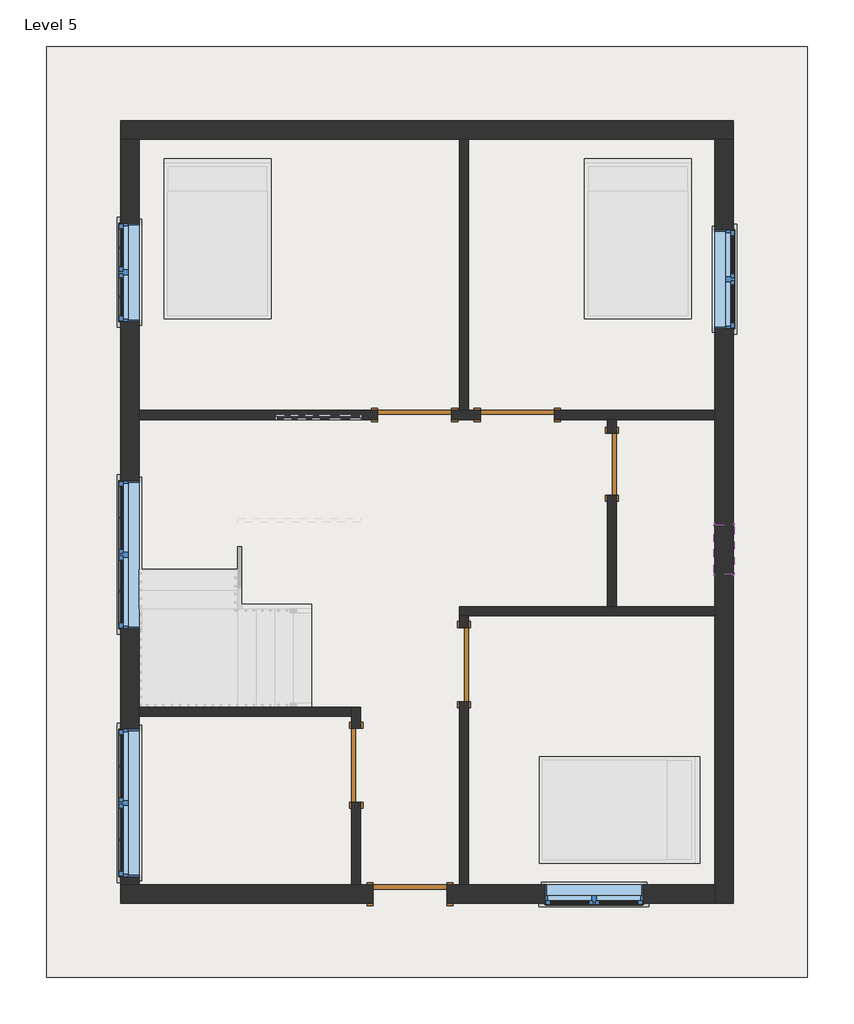
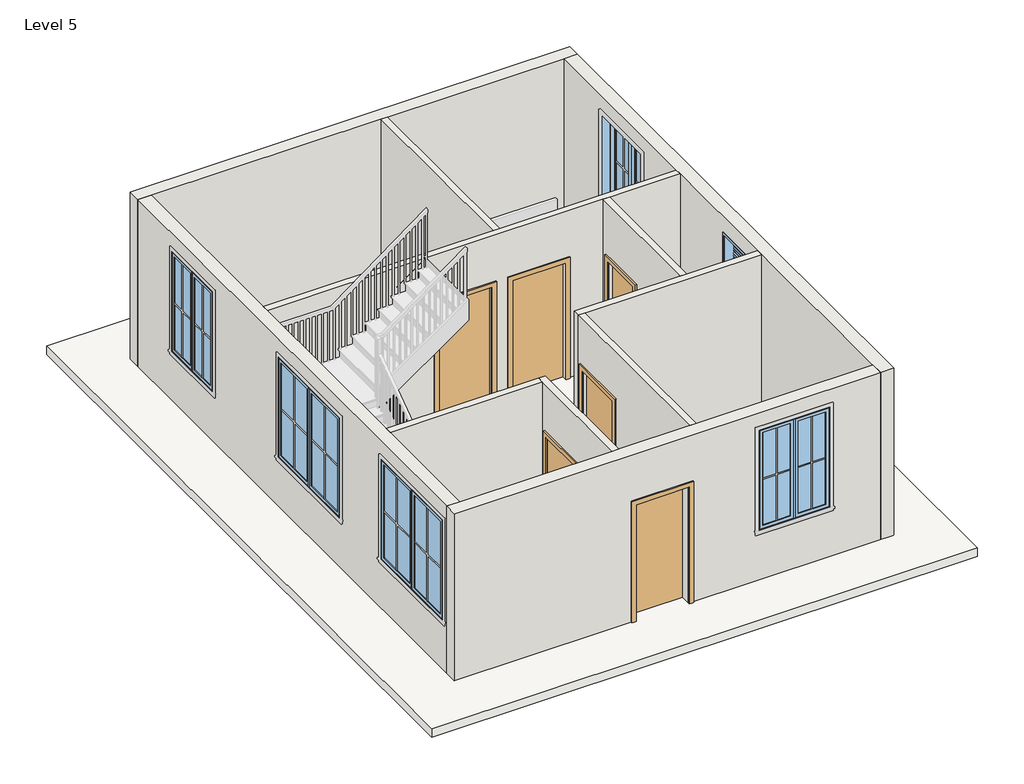
# One storey, part 1 of 3: 11 walls, 6 doors, 6 windows, 1 roof.
"""IFC4 building model written with IfcOpenShell, lengths in millimetres."""

from ifc_helpers import new_model, si_unit, frame, origin, place, context, project, spatial, polyline, outline, extrude, faceted_brep, transform, mapped, element, save
from components import door_f2b275c1, single_flush_door_3_e5f9f3c4, single_flush_door_3_305aa2a5, single_flush_door_3_a90ba1ad, window_casement_double_win_4_6ca1769e, window_casement_double_win_6_ce442eab, window_f2d8fef0

model = new_model("IFC4")

# Units and contexts
model_context = context("Model", 3, world=origin())
ifc_project = project(units=[si_unit("LENGTHUNIT", "METRE", prefix="MILLI")], contexts=[model_context])

# Site, building, storey
site = spatial("IfcSite", under=ifc_project)
building = spatial("IfcBuilding", under=site)
storey = spatial("IfcBuildingStorey", under=building, Name="Level 5", Elevation=12649.2)

# Doors
placement = place(None, origin())
door_shape = door_f2b275c1(model_context)
element("IfcDoor", 1, ObjectType="Single-Flush : 2'6\"", at=placement, inside=storey, context=model_context, shape_type="MappedRepresentation", body=[
    mapped(door_shape, transform((1031.6394609, 262.5126239, 12649.2), x_axis=(0.0, 1.0, 0.0), y_axis=(-1.0, 0.0, 0.0), z_axis=(0.0, 0.0, 1.0))),
])
single_flush_door_3_shape = single_flush_door_3_e5f9f3c4(model_context)
element("IfcDoor", 2, ObjectType="Single-Flush : door 3'", at=placement, inside=storey, context=model_context, shape_type="MappedRepresentation", body=[
    mapped(single_flush_door_3_shape, transform((-1406.7605391, 872.1126239, 12649.2), x_axis=(1.0, 0.0, 0.0), y_axis=(0.0, 1.0, 0.0), z_axis=(0.0, 0.0, 1.0))),
])
element("IfcDoor", 3, ObjectType="Single-Flush : door 3'", at=placement, inside=storey, context=model_context, shape_type="MappedRepresentation", body=[
    mapped(single_flush_door_3_shape, transform((-2130.6605391, -3458.5873761, 12649.2), x_axis=(0.0, 1.0, 0.0), y_axis=(-1.0, 0.0, 0.0), z_axis=(0.0, 0.0, 1.0))),
])
single_flush_door_3_2_shape = single_flush_door_3_305aa2a5(model_context)
element("IfcDoor", 4, ObjectType="Single-Flush : door 3'", at=placement, inside=storey, context=model_context, shape_type="MappedRepresentation", body=[
    mapped(single_flush_door_3_2_shape, transform((-136.7605391, 872.1126239, 12649.2), x_axis=(-1.0, 0.0, 0.0), y_axis=(0.0, -1.0, 0.0), z_axis=(0.0, 0.0, 1.0))),
])
element("IfcDoor", 5, ObjectType="Single-Flush : door 3'", at=placement, inside=storey, context=model_context, shape_type="MappedRepresentation", body=[
    mapped(single_flush_door_3_2_shape, transform((-797.1605391, -2213.9873761, 12649.2), x_axis=(0.0, 1.0, 0.0), y_axis=(-1.0, 0.0, 0.0), z_axis=(0.0, 0.0, 1.0))),
])
single_flush_door_3_3_shape = single_flush_door_3_a90ba1ad(model_context)
element("IfcDoor", 6, ObjectType="Single-Flush : door 3'", at=placement, inside=storey, context=model_context, shape_type="MappedRepresentation", body=[
    mapped(single_flush_door_3_3_shape, transform((-1463.9105391, -5052.4373761, 12649.2), x_axis=(-1.0, 0.0, 0.0), y_axis=(0.0, -1.0, 0.0), z_axis=(0.0, 0.0, 1.0))),
])

# Roof
element("IfcRoof", 7, ObjectType="Generic - 12\"", at=placement, inside=storey, context=model_context, shape_type="SweptSolid", body=[
    extrude(outline(polyline([(-5959.7105391, 5425.0626239), (3450.9894609, 5425.0626239), (3450.9894609, -6081.1373761), (-5959.7105391, -6081.1373761), (-5959.7105391, 5425.0626239)])), frame((0.0, 0.0, 12496.8), z_axis=(0.0, 0.0, 1.0), x_axis=(1.0, 0.0, 0.0)), (0.0, 0.0, 1.0), 152.4),
])

# Walls
element("IfcWall", 8, ObjectType="WALL 4.5\"", at=placement, inside=storey, context=model_context, shape_type="SweptSolid", body=[
    extrude(outline(polyline([(-854.3105391, 929.2626239), (-854.3105391, 4282.0626239), (-740.0105391, 4282.0626239), (-740.0105391, 929.2626239), (-854.3105391, 929.2626239)])), frame((0.0, 0.0, 12649.2), z_axis=(0.0, 0.0, 1.0), x_axis=(1.0, 0.0, 0.0)), (0.0, 0.0, 1.0), 3048.0),
])
element("IfcWall", 9, ObjectType="WALL 4.5\"", at=placement, inside=storey, context=model_context, shape_type="Brep", body=[
    faceted_brep([(-949.5605391, 814.9626239, 12649.2), (-593.9605391, 814.9626239, 12649.2), (-593.9605391, 814.9626239, 14782.8), (320.4394609, 814.9626239, 14782.8), (320.4394609, 814.9626239, 12649.2), (974.4894609, 814.9626239, 12649.2), (1088.7894609, 814.9626239, 12649.2), (2307.9894609, 814.9626239, 12649.2), (2307.9894609, 814.9626239, 15697.2), (1088.7894609, 814.9626239, 15697.2), (974.4894609, 814.9626239, 15697.2), (-4816.7105391, 814.9626239, 15697.2), (-4816.7105391, 814.9626239, 12649.2), (-1863.9605391, 814.9626239, 12649.2), (-1863.9605391, 814.9626239, 14782.8), (-949.5605391, 814.9626239, 14782.8), (-593.9605391, 929.2626239, 14782.8), (-593.9605391, 929.2626239, 12649.2), (-740.0105391, 929.2626239, 12649.2), (-854.3105391, 929.2626239, 12649.2), (-949.5605391, 929.2626239, 12649.2), (-949.5605391, 929.2626239, 14782.8), (-1863.9605391, 929.2626239, 14782.8), (-1863.9605391, 929.2626239, 12649.2), (-4816.7105391, 929.2626239, 12649.2), (-4816.7105391, 929.2626239, 15697.2), (-854.3105391, 929.2626239, 15697.2), (-740.0105391, 929.2626239, 15697.2), (2307.9894609, 929.2626239, 15697.2), (2307.9894609, 929.2626239, 12649.2), (320.4394609, 929.2626239, 12649.2), (320.4394609, 929.2626239, 14782.8)], [[[0, 1, 2, 3, 4, 5, 6, 7, 8, 9, 10, 11, 12, 13, 14, 15]], [[16, 17, 18, 19, 20, 21, 22, 23, 24, 25, 26, 27, 28, 29, 30, 31]], [[13, 12, 24, 23]], [[30, 29, 7, 6, 5, 4]], [[20, 19, 18, 17, 1, 0]], [[8, 7, 29, 28]], [[12, 11, 25, 24]], [[21, 20, 0, 15]], [[22, 21, 15, 14]], [[23, 22, 14, 13]], [[2, 1, 17, 16]], [[3, 2, 16, 31]], [[4, 3, 31, 30]], [[11, 10, 9, 8, 28, 27, 26, 25]]]),
])
element("IfcWall", 10, ObjectType="WALL 4.5\"", at=placement, inside=storey, context=model_context, shape_type="SweptSolid", body=[
    extrude(outline(polyline([(814.9626239, 12649.2), (643.5126239, 12649.2), (643.5126239, 14681.2), (-118.4873761, 14681.2), (-118.4873761, 12649.2), (-1496.4373761, 12649.2), (-1496.4373761, 15697.2), (814.9626239, 15697.2), (814.9626239, 12649.2)])), frame((974.4894609, 0.0, 0.0), z_axis=(1.0, 0.0, 0.0), x_axis=(0.0, 1.0, 0.0)), (0.0, 0.0, 1.0), 114.3),
])
element("IfcWall", 11, ObjectType="WALL 4.5\"", at=placement, inside=storey, context=model_context, shape_type="Brep", body=[
    faceted_brep([(2307.9894609, -1496.4373761, 12649.2), (1088.7894609, -1496.4373761, 12649.2), (974.4894609, -1496.4373761, 12649.2), (-854.3105391, -1496.4373761, 12649.2), (-854.3105391, -1496.4373761, 15697.2), (974.4894609, -1496.4373761, 15697.2), (1088.7894609, -1496.4373761, 15697.2), (2307.9894609, -1496.4373761, 15697.2), (2307.9894609, -1610.7373761, 12649.2), (2307.9894609, -1610.7373761, 15697.2), (-740.0105391, -1610.7373761, 15697.2), (-854.3105391, -1610.7373761, 15697.2), (-854.3105391, -1610.7373761, 12649.2), (-740.0105391, -1610.7373761, 12649.2)], [[[0, 1, 2, 3, 4, 5, 6, 7]], [[8, 9, 10, 11, 12, 13]], [[3, 2, 1, 0, 8, 13, 12]], [[0, 7, 9, 8]], [[4, 3, 12, 11]], [[7, 6, 5, 4, 11, 10, 9]]]),
])
element("IfcWall", 12, ObjectType="WALL 4.5\"", at=placement, inside=storey, context=model_context, shape_type="SweptSolid", body=[
    extrude(outline(polyline([(-1610.7373761, 12649.2), (-1756.7873761, 12649.2), (-1756.7873761, 14782.8), (-2671.1873761, 14782.8), (-2671.1873761, 12649.2), (-4938.1373761, 12649.2), (-4938.1373761, 15697.2), (-1610.7373761, 15697.2), (-1610.7373761, 12649.2)])), frame((-854.3105391, 0.0, 0.0), z_axis=(1.0, 0.0, 0.0), x_axis=(0.0, 1.0, 0.0)), (0.0, 0.0, 1.0), 114.3),
])
element("IfcWall", 13, ObjectType="WALL 4.5\"", at=placement, inside=storey, context=model_context, shape_type="Brep", body=[
    faceted_brep([(-2073.5105391, -3001.3873761, 14782.8), (-2073.5105391, -3001.3873761, 12649.2), (-2073.5105391, -2741.0373761, 12649.2), (-2073.5105391, -2741.0373761, 15697.2), (-2073.5105391, -4938.1373761, 15697.2), (-2073.5105391, -4938.1373761, 12649.2), (-2073.5105391, -3915.7873761, 12649.2), (-2073.5105391, -3915.7873761, 14782.8), (-2187.8105391, -2741.0373761, 12649.2), (-2187.8105391, -2855.3373761, 12649.2), (-2187.8105391, -3001.3873761, 12649.2), (-2187.8105391, -3001.3873761, 14782.8), (-2187.8105391, -3915.7873761, 14782.8), (-2187.8105391, -3915.7873761, 12649.2), (-2187.8105391, -4938.1373761, 12649.2), (-2187.8105391, -4938.1373761, 15697.2), (-2187.8105391, -2855.3373761, 15697.2), (-2187.8105391, -2741.0373761, 15697.2)], [[[0, 1, 2, 3, 4, 5, 6, 7]], [[8, 9, 10, 11, 12, 13, 14, 15, 16, 17]], [[6, 5, 14, 13]], [[2, 1, 10, 9, 8]], [[5, 4, 15, 14]], [[3, 2, 8, 17]], [[11, 10, 1, 0]], [[12, 11, 0, 7]], [[13, 12, 7, 6]], [[4, 3, 17, 16, 15]]]),
])
element("IfcWall", 14, ObjectType="WALL 4.5\"", at=placement, inside=storey, context=model_context, shape_type="SweptSolid", body=[
    extrude(outline(polyline([(-4816.7105391, -2741.0373761), (-2187.8105391, -2741.0373761), (-2187.8105391, -2855.3373761), (-4816.7105391, -2855.3373761), (-4816.7105391, -2741.0373761)])), frame((0.0, 0.0, 12649.2), z_axis=(0.0, 0.0, 1.0), x_axis=(1.0, 0.0, 0.0)), (0.0, 0.0, 1.0), 3048.0),
])
element("IfcWall", 15, ObjectType="WALL 9\"", at=placement, inside=storey, context=model_context, shape_type="Brep", body=[
    faceted_brep([(-5045.3105391, 4282.0626239, 12649.2), (-4816.7105391, 4282.0626239, 12649.2), (-854.3105391, 4282.0626239, 12649.2), (-740.0105391, 4282.0626239, 12649.2), (2307.9894609, 4282.0626239, 12649.2), (2536.5894609, 4282.0626239, 12649.2), (2536.5894609, 4282.0626239, 15697.2), (2307.9894609, 4282.0626239, 15697.2), (-740.0105391, 4282.0626239, 15697.2), (-854.3105391, 4282.0626239, 15697.2), (-4816.7105391, 4282.0626239, 15697.2), (-5045.3105391, 4282.0626239, 15697.2), (-5045.3105391, 4510.6626239, 12649.2), (-5045.3105391, 4510.6626239, 15697.2), (2536.5894609, 4510.6626239, 15697.2), (2536.5894609, 4510.6626239, 12649.2)], [[[0, 1, 2, 3, 4, 5, 6, 7, 8, 9, 10, 11]], [[12, 13, 14, 15]], [[5, 4, 3, 2, 1, 0, 12, 15]], [[6, 5, 15, 14]], [[0, 11, 13, 12]], [[11, 10, 9, 8, 7, 6, 14, 13]]]),
])
element("IfcWall", 16, ObjectType="WALL 9\"", at=placement, inside=storey, context=model_context, shape_type="Brep", body=[
    faceted_brep([(2307.9894609, 4282.0626239, 12649.2), (2307.9894609, 929.2626239, 12649.2), (2307.9894609, 814.9626239, 12649.2), (2307.9894609, -1496.4373761, 12649.2), (2307.9894609, -1610.7373761, 12649.2), (2307.9894609, -4938.1373761, 12649.2), (2307.9894609, -5166.7373761, 12649.2), (2307.9894609, -5166.7373761, 15697.2), (2307.9894609, -4938.1373761, 15697.2), (2307.9894609, -1610.7373761, 15697.2), (2307.9894609, -1496.4373761, 15697.2), (2307.9894609, 814.9626239, 15697.2), (2307.9894609, 929.2626239, 15697.2), (2307.9894609, 4282.0626239, 15697.2), (2307.9894609, 1938.9126239, 15392.4), (2307.9894609, 1938.9126239, 13563.6), (2307.9894609, 3158.1126239, 13563.6), (2307.9894609, 3158.1126239, 15392.4), (2307.9894609, -486.7873761, 15392.4), (2307.9894609, -1096.3873761, 15392.4), (2307.9894609, -1096.3873761, 14782.8), (2307.9894609, -486.7873761, 14782.8), (2536.5894609, 4282.0626239, 12649.2), (2536.5894609, 4282.0626239, 15697.2), (2536.5894609, -5166.7373761, 15697.2), (2536.5894609, -5166.7373761, 12649.2), (2536.5894609, 1938.9126239, 15392.4), (2536.5894609, 3158.1126239, 15392.4), (2536.5894609, 3158.1126239, 13563.6), (2536.5894609, 1938.9126239, 13563.6), (2536.5894609, -486.7873761, 15392.4), (2536.5894609, -486.7873761, 14782.8), (2536.5894609, -1096.3873761, 14782.8), (2536.5894609, -1096.3873761, 15392.4)], [[[0, 1, 2, 3, 4, 5, 6, 7, 8, 9, 10, 11, 12, 13], [14, 15, 16, 17], [18, 19, 20, 21]], [[22, 23, 24, 25], [26, 27, 28, 29], [30, 31, 32, 33]], [[6, 5, 4, 3, 2, 1, 0, 22, 25]], [[0, 13, 23, 22]], [[7, 6, 25, 24]], [[15, 14, 26, 29]], [[16, 15, 29, 28]], [[17, 16, 28, 27]], [[14, 17, 27, 26]], [[31, 30, 18, 21]], [[32, 31, 21, 20]], [[33, 32, 20, 19]], [[30, 33, 19, 18]], [[13, 12, 11, 10, 9, 8, 7, 24, 23]]]),
])
element("IfcWall", 17, ObjectType="WALL 9\"", at=placement, inside=storey, context=model_context, shape_type="Brep", body=[
    faceted_brep([(-1921.1105391, -4938.1373761, 14782.8), (-1921.1105391, -4938.1373761, 12649.2), (-2073.5105391, -4938.1373761, 12649.2), (-2187.8105391, -4938.1373761, 12649.2), (-4816.7105391, -4938.1373761, 12649.2), (-5045.3105391, -4938.1373761, 12649.2), (-5045.3105391, -4938.1373761, 15697.2), (-4816.7105391, -4938.1373761, 15697.2), (-2187.8105391, -4938.1373761, 15697.2), (-2073.5105391, -4938.1373761, 15697.2), (-854.3105391, -4938.1373761, 15697.2), (-740.0105391, -4938.1373761, 15697.2), (2307.9894609, -4938.1373761, 15697.2), (2307.9894609, -4938.1373761, 12649.2), (-740.0105391, -4938.1373761, 12649.2), (-854.3105391, -4938.1373761, 12649.2), (-1006.7105391, -4938.1373761, 12649.2), (-1006.7105391, -4938.1373761, 14782.8), (202.9644609, -4938.1373761, 15392.4), (202.9644609, -4938.1373761, 13563.6), (1422.1644609, -4938.1373761, 13563.6), (1422.1644609, -4938.1373761, 15392.4), (-5045.3105391, -5166.7373761, 12649.2), (-1921.1105391, -5166.7373761, 12649.2), (-1921.1105391, -5166.7373761, 14782.8), (-1006.7105391, -5166.7373761, 14782.8), (-1006.7105391, -5166.7373761, 12649.2), (2307.9894609, -5166.7373761, 12649.2), (2307.9894609, -5166.7373761, 15697.2), (-5045.3105391, -5166.7373761, 15697.2), (202.9644609, -5166.7373761, 15392.4), (1422.1644609, -5166.7373761, 15392.4), (1422.1644609, -5166.7373761, 13563.6), (202.9644609, -5166.7373761, 13563.6)], [[[0, 1, 2, 3, 4, 5, 6, 7, 8, 9, 10, 11, 12, 13, 14, 15, 16, 17], [18, 19, 20, 21]], [[22, 23, 24, 25, 26, 27, 28, 29], [30, 31, 32, 33]], [[5, 4, 3, 2, 1, 23, 22]], [[16, 15, 14, 13, 27, 26]], [[13, 12, 28, 27]], [[6, 5, 22, 29]], [[19, 18, 30, 33]], [[20, 19, 33, 32]], [[21, 20, 32, 31]], [[18, 21, 31, 30]], [[24, 23, 1, 0]], [[25, 24, 0, 17]], [[26, 25, 17, 16]], [[12, 11, 10, 9, 8, 7, 6, 29, 28]]]),
])
element("IfcWall", 18, ObjectType="WALL 9\"", at=placement, inside=storey, context=model_context, shape_type="Brep", body=[
    faceted_brep([(-4816.7105391, -4938.1373761, 12649.2), (-4816.7105391, -2855.3373761, 12649.2), (-4816.7105391, -2741.0373761, 12649.2), (-4816.7105391, 814.9626239, 12649.2), (-4816.7105391, 929.2626239, 12649.2), (-4816.7105391, 4282.0626239, 12649.2), (-4816.7105391, 4282.0626239, 15697.2), (-4816.7105391, 929.2626239, 15697.2), (-4816.7105391, 814.9626239, 15697.2), (-4816.7105391, -2741.0373761, 15697.2), (-4816.7105391, -2855.3373761, 15697.2), (-4816.7105391, -4938.1373761, 15697.2), (-4816.7105391, -3010.9123761, 15392.4), (-4816.7105391, -3010.9123761, 13563.6), (-4816.7105391, -4839.7123761, 13563.6), (-4816.7105391, -4839.7123761, 15392.4), (-4816.7105391, 59.3126239, 15392.4), (-4816.7105391, 59.3126239, 13563.6), (-4816.7105391, -1769.4873761, 13563.6), (-4816.7105391, -1769.4873761, 15392.4), (-4816.7105391, 3243.8376239, 15392.4), (-4816.7105391, 3243.8376239, 13563.6), (-4816.7105391, 2024.6376239, 13563.6), (-4816.7105391, 2024.6376239, 15392.4), (-5045.3105391, -4938.1373761, 12649.2), (-5045.3105391, -4938.1373761, 15697.2), (-5045.3105391, 4282.0626239, 15697.2), (-5045.3105391, 4282.0626239, 12649.2), (-5045.3105391, -3010.9123761, 15392.4), (-5045.3105391, -4839.7123761, 15392.4), (-5045.3105391, -4839.7123761, 13563.6), (-5045.3105391, -3010.9123761, 13563.6), (-5045.3105391, 59.3126239, 15392.4), (-5045.3105391, -1769.4873761, 15392.4), (-5045.3105391, -1769.4873761, 13563.6), (-5045.3105391, 59.3126239, 13563.6), (-5045.3105391, 3243.8376239, 15392.4), (-5045.3105391, 2024.6376239, 15392.4), (-5045.3105391, 2024.6376239, 13563.6), (-5045.3105391, 3243.8376239, 13563.6)], [[[0, 1, 2, 3, 4, 5, 6, 7, 8, 9, 10, 11], [12, 13, 14, 15], [16, 17, 18, 19], [20, 21, 22, 23]], [[24, 25, 26, 27], [28, 29, 30, 31], [32, 33, 34, 35], [36, 37, 38, 39]], [[5, 4, 3, 2, 1, 0, 24, 27]], [[6, 5, 27, 26]], [[0, 11, 25, 24]], [[13, 12, 28, 31]], [[14, 13, 31, 30]], [[15, 14, 30, 29]], [[12, 15, 29, 28]], [[17, 16, 32, 35]], [[18, 17, 35, 34]], [[19, 18, 34, 33]], [[16, 19, 33, 32]], [[21, 20, 36, 39]], [[22, 21, 39, 38]], [[23, 22, 38, 37]], [[20, 23, 37, 36]], [[11, 10, 9, 8, 7, 6, 26, 25]]]),
])

# Windows
window_casement_double_win_4_shape = window_casement_double_win_4_6ca1769e(model_context)
element("IfcWindow", 19, ObjectType="Window-Casement-Double : win 4'", at=placement, inside=storey, context=model_context, shape_type="MappedRepresentation", body=[
    mapped(window_casement_double_win_4_shape, transform((812.5644609, -5052.4373761, 12649.2), x_axis=(-1.0, 0.0, 0.0), y_axis=(0.0, -1.0, 0.0), z_axis=(0.0, 0.0, 1.0))),
])
element("IfcWindow", 20, ObjectType="Window-Casement-Double : win 4'", at=placement, inside=storey, context=model_context, shape_type="MappedRepresentation", body=[
    mapped(window_casement_double_win_4_shape, transform((2422.2894609, 2548.5126239, 12649.2), x_axis=(0.0, -1.0, 0.0), y_axis=(1.0, 0.0, 0.0), z_axis=(0.0, 0.0, 1.0))),
])
element("IfcWindow", 21, ObjectType="Window-Casement-Double : win 4'", at=placement, inside=storey, context=model_context, shape_type="MappedRepresentation", body=[
    mapped(window_casement_double_win_4_shape, transform((-4931.0105391, 2634.2376239, 12649.2), x_axis=(0.0, 1.0, 0.0), y_axis=(-1.0, 0.0, 0.0), z_axis=(0.0, 0.0, 1.0))),
])
window_casement_double_win_6_shape = window_casement_double_win_6_ce442eab(model_context)
element("IfcWindow", 22, ObjectType="Window-Casement-Double : win 6'", at=placement, inside=storey, context=model_context, shape_type="MappedRepresentation", body=[
    mapped(window_casement_double_win_6_shape, transform((-4931.0105391, -3925.3123761, 12649.2), x_axis=(0.0, 1.0, 0.0), y_axis=(-1.0, 0.0, 0.0), z_axis=(0.0, 0.0, 1.0))),
])
element("IfcWindow", 23, ObjectType="Window-Casement-Double : win 6'", at=placement, inside=storey, context=model_context, shape_type="MappedRepresentation", body=[
    mapped(window_casement_double_win_6_shape, transform((-4931.0105391, -855.0873761, 12649.2), x_axis=(0.0, 1.0, 0.0), y_axis=(-1.0, 0.0, 0.0), z_axis=(0.0, 0.0, 1.0))),
])
window_shape = window_f2d8fef0(model_context)
element("IfcWindow", 24, ObjectType="Window-Louvers : 24\" x 24\"", at=placement, inside=storey, context=model_context, shape_type="MappedRepresentation", body=[
    mapped(window_shape, transform((2428.6394609, -791.5873761, 13868.4), x_axis=(0.0, -1.0, 0.0), y_axis=(1.0, 0.0, 0.0), z_axis=(0.0, 0.0, 1.0))),
])

save(model, "model.ifc")

# Revit data of these elements
# Type "Single-Flush : 2'6\""
#   Type Mark = "9"
#   Construction Type Id = "MDOOR"
#   Assembly Code = "C1020"
#   Analytic Construction = "Metal"
#   Thickness = 0' - 2"
#   Heat Transfer Coefficient (U) = 0.651978 BTU/(h·ft²·°F)
#   Height = 6' - 8"
#   Trim Projection Ext = 0' - 1"
#   Trim Projection Int = 0' - 1"
#   Trim Width = 0' - 3"
#   Width = 2' - 6"
#   Define Thermal Properties by = 1
#   Door Material = Door - Panel
#   Frame Material = Door - Frame
#   Visual Light Transmittance = 0
#   Solar Heat Gain Coefficient = 0
#   Function = (empty or 0)
#   Wall Closure = (empty or 0)
# Type "Single-Flush : door 3'"
#   Type Mark = "8"
#   Construction Type Id = "MDOOR"
#   Assembly Code = "C1020"
#   Analytic Construction = "Metal"
#   Thickness = 0' - 2"
#   Heat Transfer Coefficient (U) = 0.651978 BTU/(h·ft²·°F)
#   Height = 7' - 0"
#   Trim Projection Ext = 0' - 1"
#   Trim Projection Int = 0' - 1"
#   Trim Width = 0' - 3"
#   Width = 3' - 0"
#   Define Thermal Properties by = 1
#   Door Material = Door - Panel
#   Frame Material = Door - Frame
#   Visual Light Transmittance = 0
#   Solar Heat Gain Coefficient = 0
#   Function = (empty or 0)
#   Wall Closure = (empty or 0)
# Type "Generic - 12\""
#   Assembly Code = "B1020"
#   Layers, outside or top first: 0' - 6" no material (function 1)
# Type "WALL 4.5\""
#   Assembly Code = "B2010"
#   Layers, outside or top first: 0' - 4 1/2" no material (function 1)
# Type "WALL 9\""
#   Assembly Code = "B2010"
#   Layers, outside or top first: 0' - 9" no material (function 1)
# Type "Window-Casement-Double : win 4'"
#   Type Mark = "19"
#   Fire Rating = "0.5h"
#   Assembly Code = "B2020100"
#   Analytic Construction = "Double glazing - domestic"
#   Frame Extension [instance default] = 0' - 0 1/4"
#   Window Inset [instance default] = 0' - 0"
#   Wall Thickness [instance default] = 0' - 6"
#   Interior Wall Closure [instance default] = 0' - 2 1/4"
#   Half Width = 2' - 0"
#   Visual Light Transmittance = 0.81
#   Thermal Resistance (R) = 1.8146 (h·ft²·°F)/BTU
#   Solar Heat Gain Coefficient = 0.76
#   Rough Width = 4' - 0 1/2"
#   Rough Height = 6' - 0 1/2"
#   Height = 6' - 0"
#   Heat Transfer Coefficient (U) = 0.5511 BTU/(h·ft²·°F)
#   Exterior Wall Closure [instance default] = 0' - 1 1/4"
#   Extension Jamb [instance default] = 0' - 2 1/4"
#   Default Sill Height = 3' - 0"
#   Width = 4' - 0"
#   Muntin Visibility = yes
#   Interior Trim Visibility [instance default] = yes
#   Exterior Trim Visibility [instance default] = yes
#   Extension Jamb Visibility [instance default] = yes
#   Interior Trim Material = Wood - Stained
#   Muntin Pattern = Muntin Pattern_2x2 : Muntin Pattern_2x2
#   Interior Trim = Trim-Window-Interior-Flat : Picture Frame
#   Interior Frame Material = Wood - Stained
#   Glass Panel Material = Glass
#   Exterior Trim Material = Clad - White
#   Exterior Trim = Trim-Window-Exterior-Flat : with Sill
#   Exterior Frame Material = Clad - White
#   Wall Closure = (empty or 0)
# Type "Window-Casement-Double : win 6'"
#   Type Mark = "18"
#   Fire Rating = "0.5h"
#   Assembly Code = "B2020100"
#   Analytic Construction = "Double glazing - domestic"
#   Frame Extension [instance default] = 0' - 0 1/4"
#   Window Inset [instance default] = 0' - 0"
#   Wall Thickness [instance default] = 0' - 6"
#   Interior Wall Closure [instance default] = 0' - 2 1/4"
#   Half Width = 3' - 0"
#   Visual Light Transmittance = 0.81
#   Thermal Resistance (R) = 1.8146 (h·ft²·°F)/BTU
#   Solar Heat Gain Coefficient = 0.76
#   Rough Width = 6' - 0 1/2"
#   Rough Height = 6' - 0 1/2"
#   Height = 6' - 0"
#   Heat Transfer Coefficient (U) = 0.5511 BTU/(h·ft²·°F)
#   Exterior Wall Closure [instance default] = 0' - 1 1/4"
#   Extension Jamb [instance default] = 0' - 2 1/4"
#   Default Sill Height = 3' - 0"
#   Width = 6' - 0"
#   Muntin Visibility = yes
#   Interior Trim Visibility [instance default] = yes
#   Exterior Trim Visibility [instance default] = yes
#   Extension Jamb Visibility [instance default] = yes
#   Interior Trim Material = Wood - Stained
#   Muntin Pattern = Muntin Pattern_2x2 : Muntin Pattern_2x2
#   Interior Trim = Trim-Window-Interior-Flat : Picture Frame
#   Interior Frame Material = Wood - Stained
#   Glass Panel Material = Glass
#   Exterior Trim Material = Clad - White
#   Exterior Trim = Trim-Window-Exterior-Flat : with Sill
#   Exterior Frame Material = Clad - White
#   Wall Closure = (empty or 0)
# Type "Window-Louvers : 24\" x 24\""
#   Type Mark = "20"
#   Construction Type Id = "GSP4R"
#   Assembly Code = "B20"
#   Analytic Construction = "1/8 in Pilkington single glazing"
#   Visual Light Transmittance = 0.9
#   Thermal Resistance (R) = 1.53941 (h·ft²·°F)/BTU
#   Solar Heat Gain Coefficient = 0.78
#   Max Height = 1' - 11.74264"
#   Height = 2' - 0"
#   Heat Transfer Coefficient (U) = 0.6496 BTU/(h·ft²·°F)
#   Blade Width [instance default] = 1' - 10 1/2"
#   Blade Vertical Thickness = 0' - 0.35355"
#   Blade Thickness = 0' - 0 1/4"
#   Blade Spacing = 0' - 1 1/2"
#   Blade Height = 0' - 1.85355"
#   Blade Depth = 0' - 3"
#   Blade Angle = 45.00°
#   Default Sill Height = 3' - 0"
#   Trim Projection_Exterior = 0' - 0 1/2"
#   Trim Projection_Interior = 0' - 0 1/2"
#   Trim Width_Exterior = 0' - 1 1/2"
#   Trim Width_Interior = 0' - 1 1/2"
#   Width = 2' - 0"
#   Max Blade Count = 12
#   Define Thermal Properties by = 1
#   Blade Count = 12
#   Frame Material = Birch
#   Louver Material = Birch
#   Trim Exterior Material = Birch
#   Trim Interior Material = Birch
#   Wall Closure = (empty or 0)
# Element 1 (IfcDoor, "Single-Flush : 2'6\"")
#   Phase Created = New Construction
#   Materials on its faces: "Door - Frame", "Door - Panel"
# Elements 2, 3, 4, 5, 6 (IfcDoor, "Single-Flush : door 3'")
#   Phase Created = New Construction
#   Materials on its faces: "Door - Frame", "Door - Panel"
# Element 7 (IfcRoof, "Generic - 12\"")
#   built-in parameter 1001705 = 41.5 (stored number, unit not read)
#   built-in parameter 1001701 = -0.5 (stored number, unit not read)
#   built-in parameter 1001710 = 33615
#   Phase Created = New Construction
#   Materials on its faces: "Wood Planks", "Wood - Stained"
# Elements 8, 9, 10, 11, 12, 13, 14 (IfcWall, "WALL 4.5\"")
#   Top Offset = 0' - 0"
#   Base Offset = 0' - 0"
#   Unconnected Height = 10' - 0"
#   wall height = 10' - 0"
#   Phase Created = New Construction
#   Base Constraint = Level 5
#   Materials on its faces: "Default Wall"
# Elements 15, 16, 17, 18 (IfcWall, "WALL 9\"")
#   Top Offset = 0' - 0"
#   Base Offset = 0' - 0"
#   Unconnected Height = 10' - 0"
#   wall height = 10' - 0"
#   Phase Created = New Construction
#   Base Constraint = Level 5
#   Materials on its faces: "Default Wall", "Door - Frame"
# Element 19 (IfcWindow, "Window-Casement-Double : win 4'")
#   Mark = "27"
#   Window Inset = 0' - 0"
#   Interior Wall Closure = 0' - 2 1/4"
#   Frame Extension = 0' - 0 1/4"
#   Exterior Wall Closure = 0' - 1 1/4"
#   Interior Trim Visibility = yes
#   Exterior Trim Visibility = yes
#   Phase Created = New Construction
#   Materials on its faces: "Wood - Stained", "Glass", "Clad - White"
# Element 20 (IfcWindow, "Window-Casement-Double : win 4'")
#   Mark = "28"
#   Window Inset = 0' - 0"
#   Interior Wall Closure = 0' - 2 1/4"
#   Frame Extension = 0' - 0 1/4"
#   Exterior Wall Closure = 0' - 1 1/4"
#   Interior Trim Visibility = yes
#   Exterior Trim Visibility = yes
#   Phase Created = New Construction
#   Materials on its faces: "Wood - Stained", "Glass", "Clad - White"
# Element 21 (IfcWindow, "Window-Casement-Double : win 4'")
#   Mark = "29"
#   Window Inset = 0' - 0"
#   Interior Wall Closure = 0' - 2 1/4"
#   Frame Extension = 0' - 0 1/4"
#   Exterior Wall Closure = 0' - 1 1/4"
#   Interior Trim Visibility = yes
#   Exterior Trim Visibility = yes
#   Phase Created = New Construction
#   Materials on its faces: "Wood - Stained", "Glass", "Clad - White"
# Element 22 (IfcWindow, "Window-Casement-Double : win 6'")
#   Mark = "25"
#   Window Inset = 0' - 0"
#   Interior Wall Closure = 0' - 2 1/4"
#   Frame Extension = 0' - 0 1/4"
#   Exterior Wall Closure = 0' - 1 1/4"
#   Interior Trim Visibility = yes
#   Exterior Trim Visibility = yes
#   Phase Created = New Construction
#   Materials on its faces: "Wood - Stained", "Glass", "Clad - White"
# Element 23 (IfcWindow, "Window-Casement-Double : win 6'")
#   Mark = "26"
#   Window Inset = 0' - 0"
#   Interior Wall Closure = 0' - 2 1/4"
#   Frame Extension = 0' - 0 1/4"
#   Exterior Wall Closure = 0' - 1 1/4"
#   Interior Trim Visibility = yes
#   Exterior Trim Visibility = yes
#   Phase Created = New Construction
#   Materials on its faces: "Wood - Stained", "Glass", "Clad - White"
# Element 24 (IfcWindow, "Window-Louvers : 24\" x 24\"")
#   Mark = "30"
#   Blade Width = 1' - 10 1/2"
#   Phase Created = New Construction
#   Materials on its faces: "Birch"
# Materials
#   "Door - Panel": class "Wood", colour RGB 210 159 95, transparency 0, Cost = 0
#   "Door - Frame": colour RGB 118 70 51, transparency 0, Cost = 0
#   "Wood - Stained": class "Wood", colour RGB 224 178 126, transparency 0, Cost = 0
#   "Glass": class "Glass", colour RGB 0 128 192, transparency 0.75, Description = "Soda Lime Glass", Cost = 0
#   "Clad - White": class "Wood", colour RGB 242 242 238, transparency 0, Cost = 0
#   "Birch": class "Wood", colour RGB 224 178 126, transparency 0, Description = "Betula Alleghaniensis", Cost = 0
#   "Wood Planks": class "Wood", colour RGB 193 160 115, transparency 0, Description = "Physical material.", Cost = 0
#   "Default Wall": colour RGB 128 128 128, transparency 0, Cost = 0
